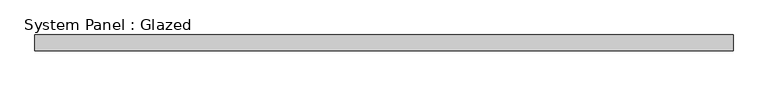
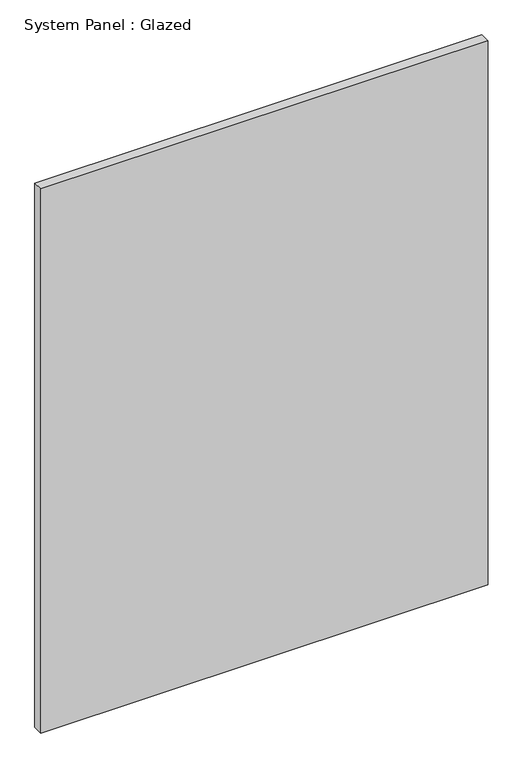
"""IFC4 building model written with IfcOpenShell, lengths in millimetres: plate geometry, System Panel : Glazed."""

from ifc_helpers import new_model, si_unit, origin, origin_with_axes, place, context, project, spatial, polyline, outline, extrude, source, transform, mapped, element, save


def system_panel_glazed_448caaff(model_context):
    return source(origin(), model_context, "Body", "SweptSolid", [
        extrude(outline(polyline([(555.625, 19.05), (-555.625, 19.05), (-555.625, 44.45), (555.625, 44.45), (555.625, 19.05)])), origin_with_axes(), (0.0, 0.0, 1.0), 1428.75),
    ])


if __name__ == "__main__":
    model = new_model("IFC4")
    model_context = context("Model", 3, world=origin())
    ifc_project = project(units=[si_unit("LENGTHUNIT", "METRE", prefix="MILLI")], contexts=[model_context])
    site = spatial("IfcSite", under=ifc_project)
    building = spatial("IfcBuilding", under=site)
    placement = place(None, origin())
    system_panel_glazed_shape = system_panel_glazed_448caaff(model_context)
    element("IfcPlate", 1, ObjectType="System Panel : Glazed", at=placement, inside=building, context=model_context, shape_type="MappedRepresentation", body=[
        mapped(system_panel_glazed_shape, transform((0.0, 0.0, 0.0), x_axis=(1.0, 0.0, 0.0), y_axis=(0.0, 1.0, 0.0), z_axis=(0.0, 0.0, 1.0))),
    ])
    save(model, "model.ifc")

# Revit data of these elements
# Type "System Panel : Glazed"
#   Construction Type Id = "GSP4R"
#   Analytic Construction = "1/8 in Pilkington single glazing"
#   Visual Light Transmittance = 0.9
#   Solar Heat Gain Coefficient = 0.86
#   Heat Transfer Coefficient (U) = 1.18115 BTU/(h·ft²·°F)
#   Define Thermal Properties by = 1
# Element 1 (IfcPlate, "System Panel : Glazed")
#   Materials on its faces: "Glass"
# Materials
#   "Glass": class "Glass", colour RGB 0 128 192, transparency 0.75, Description = "Soda Lime Glass", Cost = 0
